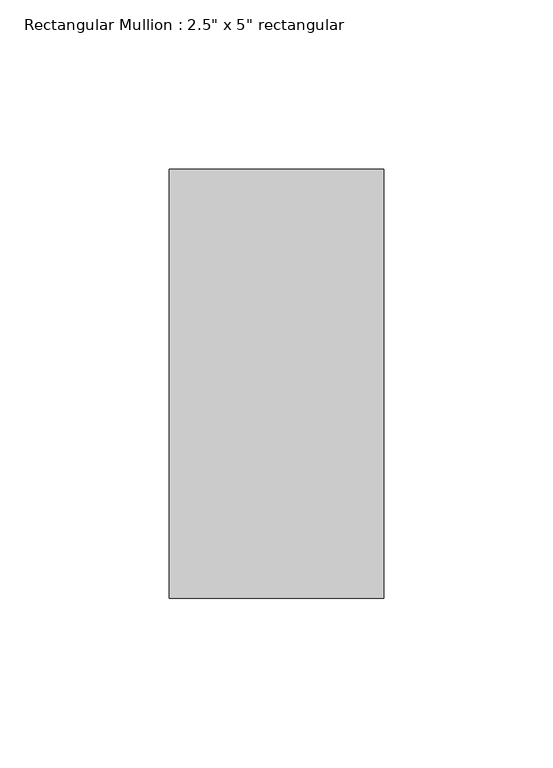
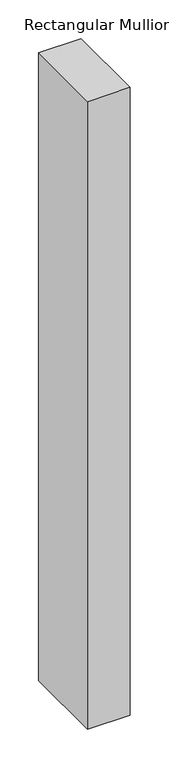
"""IFC4 building model written with IfcOpenShell, lengths in millimetres: member geometry."""

from ifc_helpers import new_model, si_unit, frame, origin, place, context, project, spatial, polyline, outline, extrude, source, transform, mapped, element, save


def member_3b0b2d0d(model_context):
    return source(origin(), model_context, "Body", "SweptSolid", [
        extrude(outline(polyline([(31.75, 63.5), (31.75, -63.5), (-31.75, -63.5), (-31.75, 63.5), (31.75, 63.5)])), frame((0.0, 0.0, -990.6), z_axis=(0.0, 0.0, 1.0), x_axis=(1.0, 0.0, 0.0)), (0.0, 0.0, 1.0), 990.6),
    ])


if __name__ == "__main__":
    model = new_model("IFC4")
    model_context = context("Model", 3, world=origin())
    ifc_project = project(units=[si_unit("LENGTHUNIT", "METRE", prefix="MILLI")], contexts=[model_context])
    site = spatial("IfcSite", under=ifc_project)
    building = spatial("IfcBuilding", under=site)
    placement = place(None, origin())
    member_shape = member_3b0b2d0d(model_context)
    element("IfcMember", 1, ObjectType="Rectangular Mullion : 2.5\" x 5\" rectangular", at=placement, inside=building, context=model_context, shape_type="MappedRepresentation", body=[
        mapped(member_shape, transform((0.0, 0.0, 0.0), x_axis=(1.0, 0.0, 0.0), y_axis=(0.0, 1.0, 0.0), z_axis=(0.0, 0.0, 1.0))),
    ])
    save(model, "model.ifc")

# Revit data of these elements
# Type "Rectangular Mullion : 2.5\" x 5\" rectangular"
#   built-in parameter 1007304 = 0.416667 (stored number, unit not read)
#   built-in parameter 1007301 = 0.104167 (stored number, unit not read)
#   built-in parameter 1007300 = 0.104167 (stored number, unit not read)
# Element 1 (IfcMember, "Rectangular Mullion : 2.5\" x 5\" rectangular")
#   Materials on its faces: "Aluminum"
# Materials
#   "Aluminum": class "Metal", colour RGB 247 247 247, transparency 0, Description = "Aluminum 6061", Cost = 0
